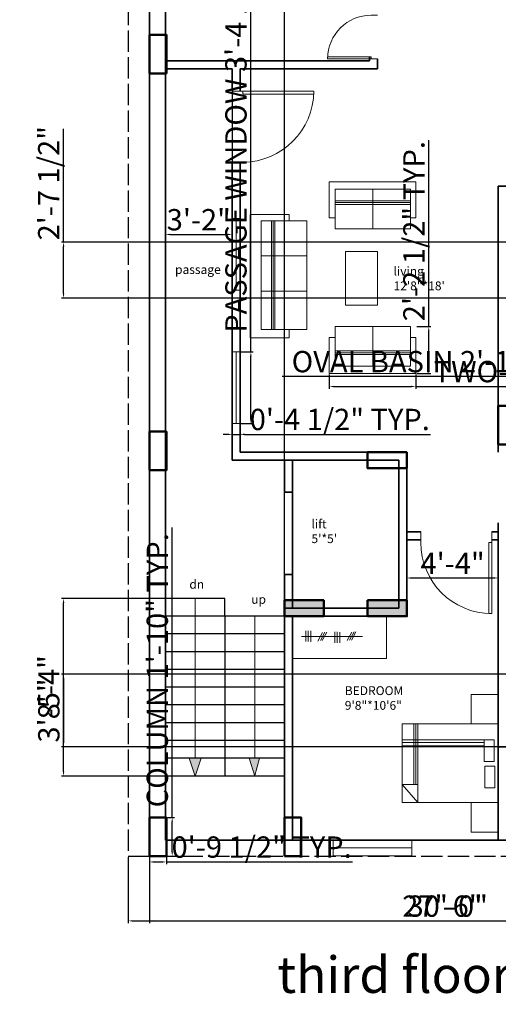
# Model space of a CAD drawing. Units: inches. Extents: x 2147 to 2722, y 2048 to 2905.
# Tile 1 of 3: x 2147 to 2417, y 2048 to 2602. Entities that reach past the tile are written whole.
import ezdxf

# ---------------------------------------------------------------- set-up
doc = ezdxf.new("R2010")
doc.units = ezdxf.units.IN
doc.linetypes.add('ACAD_ISO02W100', pattern=[15, 12, -3])
for name, color, linetype, lineweight in [('A-ANNO-DIMS', 2, 'Continuous', 18), ('A-ANNO-SYMB', 7, 'Continuous', 18), ('A-ANNO-TEXT', 7, 'Continuous', 18), ('A-ANNO-TITL', 7, 'Continuous', 35), ('A-AREA-IDEN', 7, 'Continuous', 18), ('A-COLS', 7, 'Continuous', 50), ('A-COLS-PATT', 252, 'Continuous', 13), ('A-DOOR', 3, 'Continuous', 18), ('A-FLOR-CASE', 8, 'Continuous', 18), ('A-FLOR-PATT', 252, 'Continuous', 13), ('A-FLOR-STRS', 7, 'Continuous', 25), ('A-FURN', 8, 'Continuous', 18), ('A-GLAZ', 4, 'Continuous', 18), ('A-WALL', 7, 'Continuous', 35), ('C-PROP', 6, 'ACAD_ISO02W100', 25)]:
    doc.layers.add(name, color=color, linetype=linetype, lineweight=lineweight)
doc.styles.get("Standard").update_dxf_attribs({"font": 'arial.ttf'})
doc.dimstyles.new('ISO-25', dxfattribs={"dimtxt": 12, "dimasz": 2.5, "dimexe": 1.25, "dimexo": 0.625, "dimtad": 1, "dimdec": 0, "dimlunit": 4, "dimtxsty": 'Standard', "dimcen": 2.5, "dimadec": 0, "dimazin": 0, "dimtfac": 1, "dimtdec": 0, "dimtmove": 0, "dimatfit": 3, "dimfxl": 1, "dimarcsym": 0})

# ---------------------------------------------------------------- blocks, each defined once
blk = doc.blocks.new('*U3')
for p, q in [((0, 0), (0, -6)), ((40, 0), (40, -6))]:
    blk.add_line(p, q)
blk.add_lwpolyline([(0, 0), (0, 40), (1.75, 40), (1.75, 0)], close=True)
blk.add_arc((0, 0), 40, 0, 90)
blk = doc.blocks.new('*D6')
at = {"layer": 'A-ANNO-DIMS', "color": 0, "lineweight": -2, "transparency": 16777216}
for p, q in [((2229.6, 2573.86), (2229.6, 2479.91)), ((2267.1, 2573.86), (2267.1, 2479.91)), ((2232.1, 2481.16), (2264.6, 2481.16))]:
    blk.add_line(p, q, dxfattribs=at)
at = {"layer": 'A-ANNO-DIMS', "color": 0, "lineweight": 100, "transparency": 16777216}
for points in [[(2232.1, 2481.58), (2232.1, 2480.74), (2229.6, 2481.16)], [(2264.6, 2481.58), (2264.6, 2480.74), (2267.1, 2481.16)]]:
    blk.add_solid(points, dxfattribs=at)
at = {"layer": 'Defpoints', "color": 0, "lineweight": 100, "transparency": 16777216}
for p in [(2229.6, 2574.49), (2267.1, 2574.49), (2267.1, 2481.16)]:
    blk.add_point(p, dxfattribs=at)
at = {"layer": 'A-ANNO-DIMS', "color": 0, "transparency": 16777216, "insert": (2248.35, 2487.92), "char_height": 12, "attachment_point": 5}
blk.add_mtext('3\'-2"', dxfattribs=at)
blk = doc.blocks.new('*D9')
at = {"layer": 'A-ANNO-DIMS', "color": 0, "lineweight": -2, "transparency": 16777216}
for p, q in [((2365.59, 2313.02), (2365.59, 2286.43)), ((2417.09, 2313.02), (2417.09, 2286.43)), ((2368.09, 2287.68), (2414.59, 2287.68))]:
    blk.add_line(p, q, dxfattribs=at)
at = {"layer": 'A-ANNO-DIMS', "color": 0, "lineweight": 100, "transparency": 16777216}
for points in [[(2368.09, 2288.1), (2368.09, 2287.27), (2365.59, 2287.68)], [(2414.59, 2288.1), (2414.59, 2287.27), (2417.09, 2287.68)]]:
    blk.add_solid(points, dxfattribs=at)
at = {"layer": 'Defpoints', "color": 0, "lineweight": 100, "transparency": 16777216}
for p in [(2365.59, 2313.64), (2417.09, 2313.64), (2417.09, 2287.68)]:
    blk.add_point(p, dxfattribs=at)
at = {"layer": 'A-ANNO-DIMS', "color": 0, "transparency": 16777216, "insert": (2391.34, 2294.31), "char_height": 12, "attachment_point": 5}
blk.add_mtext('4\'-4"', dxfattribs=at)
blk = doc.blocks.new('BED-TWIN-PILLOW')
for p, q in [((6.6, 10.17), (6.6, 44.18)), ((7.66, 10.17), (7.66, 44.18)), ((8.88, 10.17), (8.88, 44.18)), ((46.28, 35.34), (0, 35.34)), ((46.28, 33.66), (0, 33.66)), ((46.28, 31.83), (0, 31.83)), ((8.88, 0), (0, 10.17))]:
    blk.add_line(p, q)
for points in [[(54.22, 44.18), (0, 44.18), (0, 0), (54.22, 0)], [(51.93, 35.34), (46.28, 35.34), (46.28, 23.14), (51.93, 23.14)], [(52.24, 20.39), (46.59, 20.39), (46.59, 8.19), (52.24, 8.19)], [(0, 0), (8.88, 0), (8.88, 10.17), (0, 10.17)]]:
    blk.add_lwpolyline(points, close=True)
blk = doc.blocks.new('NIGHTSTAND')
blk.add_lwpolyline([(15.28, 0), (0, 0), (0, 16.69), (15.28, 16.69)], close=True)
blk = doc.blocks.new('SOFA-TWO-SEAT')
for p, q in [((24.52, 26.42), (24.52, 4.08)), ((3.35, 20.33), (0, 20.33)), ((0, 20.33), (0, 0)), ((48.72, 20.33), (45.68, 20.33)), ((48.72, 0), (48.72, 20.33)), ((3.35, 12.7), (45.68, 12.7)), ((3.35, 11.65), (45.68, 11.65)), ((3.35, 10.79), (45.68, 10.79)), ((0, 0), (48.72, 0))]:
    blk.add_line(p, q)
blk.add_lwpolyline([(3.35, 26.42), (45.68, 26.42), (45.68, 4.08), (3.35, 4.08)], close=True)
blk = doc.blocks.new('WINDOW-BEDROOM')
blk.add_line((0, 4.5), (44.35, 4.5))
blk.add_lwpolyline([(0, 9), (44.35, 9), (44.35, 0), (0, 0)], close=True)
blk = doc.blocks.new('WINDOW-PASSAGE')
blk.add_line((2.25, 0), (2.25, 40.45))
blk.add_lwpolyline([(0, 0), (4.5, 0), (4.5, 40.45), (0, 40.45)], close=True)
blk = doc.blocks.new('COLUMN-RECT')
blk.add_lwpolyline([(0, 0), (9.48, 0), (9.48, 21.75), (0, 21.75)], close=True)
blk = doc.blocks.new('*D26')
at = {"layer": 'A-ANNO-DIMS', "color": 0, "lineweight": -2, "transparency": 16777216}
for p, q in [((2233.34, 2152.74), (2233.34, 2316.12)), ((2230.7, 2152.74), (2234.59, 2152.74)), ((2233.34, 2133.49), (2233.34, 2150.24)), ((2230.7, 2130.99), (2234.59, 2130.99))]:
    blk.add_line(p, q, dxfattribs=at)
at = {"layer": 'A-ANNO-DIMS', "color": 0, "lineweight": 100, "transparency": 16777216}
for points in [[(2232.92, 2150.24), (2233.76, 2150.24), (2233.34, 2152.74)], [(2232.92, 2133.49), (2233.76, 2133.49), (2233.34, 2130.99)]]:
    blk.add_solid(points, dxfattribs=at)
at = {"layer": 'Defpoints', "color": 0, "lineweight": 100, "transparency": 16777216}
for p in [(2230.08, 2152.74), (2233.34, 2152.74), (2230.08, 2130.99)]:
    blk.add_point(p, dxfattribs=at)
at = {"layer": 'A-ANNO-DIMS', "color": 0, "transparency": 16777216, "insert": (2226.51, 2235.68), "char_height": 12, "attachment_point": 5, "rotation": 90}
blk.add_mtext('COLUMN 1\'-10" TYP.', dxfattribs=at)
blk = doc.blocks.new('*D27')
at = {"layer": 'A-ANNO-DIMS', "color": 0, "lineweight": -2, "transparency": 16777216}
for p, q in [((2220.6, 2130.36), (2220.6, 2126.48)), ((2230.08, 2130.36), (2230.08, 2126.48)), ((2223.1, 2127.73), (2227.58, 2127.73)), ((2230.08, 2127.73), (2334.94, 2127.73))]:
    blk.add_line(p, q, dxfattribs=at)
at = {"layer": 'A-ANNO-DIMS', "color": 0, "lineweight": 100, "transparency": 16777216}
for points in [[(2223.1, 2128.14), (2223.1, 2127.31), (2220.6, 2127.73)], [(2227.58, 2128.14), (2227.58, 2127.31), (2230.08, 2127.73)]]:
    blk.add_solid(points, dxfattribs=at)
at = {"layer": 'Defpoints', "color": 0, "lineweight": 100, "transparency": 16777216}
for p in [(2220.6, 2130.99), (2230.08, 2130.99), (2230.08, 2127.73)]:
    blk.add_point(p, dxfattribs=at)
at = {"layer": 'A-ANNO-DIMS', "color": 0, "transparency": 16777216, "insert": (2283.76, 2134.56), "char_height": 12, "attachment_point": 5}
blk.add_mtext('0\'-9 1/2" TYP.', dxfattribs=at)
blk = doc.blocks.new('*D30')
at = {"layer": 'A-ANNO-DIMS', "color": 0, "lineweight": -2, "transparency": 16777216}
for p, q in [((2476.51, 2404.28), (2476.51, 2399.9)), ((2501.53, 2404.28), (2501.53, 2399.9)), ((2476.51, 2401.15), (2295.38, 2401.15)), ((2499.03, 2401.15), (2479.01, 2401.15))]:
    blk.add_line(p, q, dxfattribs=at)
at = {"layer": 'A-ANNO-DIMS', "color": 0, "lineweight": 100, "transparency": 16777216}
for points in [[(2479.01, 2401.57), (2479.01, 2400.73), (2476.51, 2401.15)], [(2499.03, 2401.57), (2499.03, 2400.73), (2501.53, 2401.15)]]:
    blk.add_solid(points, dxfattribs=at)
at = {"layer": 'Defpoints', "color": 0, "lineweight": 100, "transparency": 16777216}
for p in [(2476.51, 2404.9), (2501.53, 2404.9), (2476.51, 2401.15)]:
    blk.add_point(p, dxfattribs=at)
at = {"layer": 'A-ANNO-DIMS', "color": 0, "transparency": 16777216, "insert": (2384.7, 2407.98), "char_height": 12, "attachment_point": 5}
blk.add_mtext('OVAL BASIN 2\'-1" TYP.', dxfattribs=at)
blk = doc.blocks.new('*D38')
at = {"layer": 'A-ANNO-DIMS', "color": 0, "lineweight": -2, "transparency": 16777216}
for p, q in [((2321.88, 2402.21), (2321.88, 2394.28)), ((2370.6, 2402.21), (2370.6, 2394.28)), ((2324.38, 2395.53), (2368.1, 2395.53)), ((2370.6, 2395.53), (2619.19, 2395.53))]:
    blk.add_line(p, q, dxfattribs=at)
at = {"layer": 'A-ANNO-DIMS', "color": 0, "lineweight": 100, "transparency": 16777216}
for points in [[(2324.38, 2395.95), (2324.38, 2395.11), (2321.88, 2395.53)], [(2368.1, 2395.95), (2368.1, 2395.11), (2370.6, 2395.53)]]:
    blk.add_solid(points, dxfattribs=at)
at = {"layer": 'Defpoints', "color": 0, "lineweight": 100, "transparency": 16777216}
for p in [(2321.88, 2402.84), (2370.6, 2402.84), (2370.6, 2395.53)]:
    blk.add_point(p, dxfattribs=at)
at = {"layer": 'A-ANNO-DIMS', "color": 0, "transparency": 16777216, "insert": (2496.15, 2402.36), "char_height": 12, "attachment_point": 5}
blk.add_mtext('TWO-SEAT SOFA 4\'-0 1/2" TYP.', dxfattribs=at)
blk = doc.blocks.new('*D39')
at = {"layer": 'A-ANNO-DIMS', "color": 0, "lineweight": -2, "transparency": 16777216}
for p, q in [((2377.91, 2429.26), (2377.91, 2534.32)), ((2371.23, 2429.26), (2379.16, 2429.26)), ((2377.91, 2405.34), (2377.91, 2426.76)), ((2371.23, 2402.84), (2379.16, 2402.84))]:
    blk.add_line(p, q, dxfattribs=at)
at = {"layer": 'A-ANNO-DIMS', "color": 0, "lineweight": 100, "transparency": 16777216}
for points in [[(2377.49, 2426.76), (2378.33, 2426.76), (2377.91, 2429.26)], [(2377.49, 2405.34), (2378.33, 2405.34), (2377.91, 2402.84)]]:
    blk.add_solid(points, dxfattribs=at)
at = {"layer": 'Defpoints', "color": 0, "lineweight": 100, "transparency": 16777216}
for p in [(2370.6, 2429.26), (2377.91, 2429.26), (2370.6, 2402.84)]:
    blk.add_point(p, dxfattribs=at)
at = {"layer": 'A-ANNO-DIMS', "color": 0, "transparency": 16777216, "insert": (2371.08, 2483.04), "char_height": 12, "attachment_point": 5, "rotation": 90}
blk.add_mtext('2\'-2 1/2" TYP.', dxfattribs=at)
blk = doc.blocks.new('*D44')
at = {"layer": 'A-ANNO-DIMS', "color": 0, "lineweight": -2, "transparency": 16777216}
for p, q in [((2277.67, 2415.1), (2277.67, 2682.36)), ((2272.22, 2415.1), (2278.92, 2415.1)), ((2277.67, 2377.15), (2277.67, 2412.6)), ((2272.22, 2374.65), (2278.92, 2374.65))]:
    blk.add_line(p, q, dxfattribs=at)
at = {"layer": 'A-ANNO-DIMS', "color": 0, "lineweight": 100, "transparency": 16777216}
for points in [[(2277.25, 2412.6), (2278.08, 2412.6), (2277.67, 2415.1)], [(2277.25, 2377.15), (2278.08, 2377.15), (2277.67, 2374.65)]]:
    blk.add_solid(points, dxfattribs=at)
at = {"layer": 'Defpoints', "color": 0, "lineweight": 100, "transparency": 16777216}
for p in [(2271.6, 2415.1), (2277.67, 2415.1), (2271.6, 2374.65)]:
    blk.add_point(p, dxfattribs=at)
at = {"layer": 'A-ANNO-DIMS', "color": 0, "transparency": 16777216, "insert": (2270.83, 2549.98), "char_height": 12, "attachment_point": 5, "rotation": 90}
blk.add_mtext('PASSAGE WINDOW 3\'-4 1/2" TYP.', dxfattribs=at)
blk = doc.blocks.new('*D45')
at = {"layer": 'A-ANNO-DIMS', "color": 0, "lineweight": -2, "transparency": 16777216}
for p, q in [((2267.1, 2374.02), (2267.1, 2367.33)), ((2271.6, 2374.02), (2271.6, 2367.33)), ((2264.6, 2368.58), (2262.1, 2368.58)), ((2267.1, 2368.58), (2271.6, 2368.58)), ((2274.1, 2368.58), (2378.95, 2368.58))]:
    blk.add_line(p, q, dxfattribs=at)
at = {"layer": 'A-ANNO-DIMS', "color": 0, "lineweight": 100, "transparency": 16777216}
for points in [[(2264.6, 2369), (2264.6, 2368.16), (2267.1, 2368.58)], [(2274.1, 2369), (2274.1, 2368.16), (2271.6, 2368.58)]]:
    blk.add_solid(points, dxfattribs=at)
at = {"layer": 'Defpoints', "color": 0, "lineweight": 100, "transparency": 16777216}
for p in [(2267.1, 2374.65), (2271.6, 2374.65), (2271.6, 2368.58)]:
    blk.add_point(p, dxfattribs=at)
at = {"layer": 'A-ANNO-DIMS', "color": 0, "transparency": 16777216, "insert": (2327.78, 2375.41), "char_height": 12, "attachment_point": 5}
blk.add_mtext('0\'-4 1/2" TYP.', dxfattribs=at)
blk = doc.blocks.new('*D46')
at = {"layer": 'A-ANNO-DIMS', "color": 0, "lineweight": -2, "transparency": 16777216}
for p, q in [((2208.6, 2130.36), (2208.6, 2093.29)), ((2568.6, 2130.36), (2568.6, 2093.29)), ((2211.1, 2094.54), (2566.1, 2094.54))]:
    blk.add_line(p, q, dxfattribs=at)
at = {"layer": 'A-ANNO-DIMS', "color": 0, "lineweight": 100, "transparency": 16777216}
for points in [[(2211.1, 2094.96), (2211.1, 2094.12), (2208.6, 2094.54)], [(2566.1, 2094.96), (2566.1, 2094.12), (2568.6, 2094.54)]]:
    blk.add_solid(points, dxfattribs=at)
at = {"layer": 'Defpoints', "color": 0, "lineweight": 100, "transparency": 16777216}
for p in [(2208.6, 2130.99), (2568.6, 2130.99), (2568.6, 2094.54)]:
    blk.add_point(p, dxfattribs=at)
at = {"layer": 'A-ANNO-DIMS', "color": 0, "transparency": 16777216, "insert": (2388.6, 2101.3), "char_height": 12, "attachment_point": 5}
blk.add_mtext('30\'-0"', dxfattribs=at)
blk = doc.blocks.new('*D47')
at = {"layer": 'A-ANNO-DIMS', "color": 0, "lineweight": -2, "transparency": 16777216}
for p, q in [((2220.6, 2130.36), (2220.6, 2093.29)), ((2550.6, 2130.51), (2550.6, 2093.29)), ((2223.1, 2094.54), (2548.1, 2094.54))]:
    blk.add_line(p, q, dxfattribs=at)
at = {"layer": 'A-ANNO-DIMS', "color": 0, "lineweight": 100, "transparency": 16777216}
for points in [[(2223.1, 2094.96), (2223.1, 2094.12), (2220.6, 2094.54)], [(2548.1, 2094.96), (2548.1, 2094.12), (2550.6, 2094.54)]]:
    blk.add_solid(points, dxfattribs=at)
at = {"layer": 'Defpoints', "color": 0, "lineweight": 100, "transparency": 16777216}
for p in [(2220.6, 2130.99), (2550.6, 2131.13), (2550.6, 2094.54)]:
    blk.add_point(p, dxfattribs=at)
at = {"layer": 'A-ANNO-DIMS', "color": 0, "transparency": 16777216, "insert": (2385.6, 2101.29), "char_height": 12, "attachment_point": 5}
blk.add_mtext('27\'-6"', dxfattribs=at)
blk = doc.blocks.new('*D48')
at = {"layer": 'A-ANNO-DIMS', "color": 0, "lineweight": -2, "transparency": 16777216}
for p, q in [((2229.6, 2266.77), (2229.6, 2768.69)), ((2232.1, 2767.44), (2294.09, 2767.44)), ((2296.59, 2266.77), (2296.59, 2768.69))]:
    blk.add_line(p, q, dxfattribs=at)
at = {"layer": 'A-ANNO-DIMS', "color": 0, "lineweight": 100, "transparency": 16777216}
for points in [[(2232.1, 2767.86), (2232.1, 2767.02), (2229.6, 2767.44)], [(2294.09, 2767.86), (2294.09, 2767.02), (2296.59, 2767.44)]]:
    blk.add_solid(points, dxfattribs=at)
at = {"layer": 'Defpoints', "color": 0, "lineweight": 100, "transparency": 16777216}
for p in [(2296.59, 2767.44), (2229.6, 2266.14), (2296.59, 2266.14)]:
    blk.add_point(p, dxfattribs=at)
at = {"layer": 'A-ANNO-DIMS', "color": 0, "transparency": 16777216, "insert": (2263.1, 2774.17), "char_height": 12, "attachment_point": 5}
blk.add_mtext('5\'-7"', dxfattribs=at)
blk = doc.blocks.new('*D49')
at = {"layer": 'A-ANNO-DIMS', "color": 0, "lineweight": -2, "transparency": 16777216}
for p, q in [((2228.97, 2276.14), (2170.9, 2276.14)), ((2172.15, 2178.64), (2172.15, 2273.64)), ((2228.97, 2176.14), (2170.9, 2176.14))]:
    blk.add_line(p, q, dxfattribs=at)
at = {"layer": 'A-ANNO-DIMS', "color": 0, "lineweight": 100, "transparency": 16777216}
for points in [[(2171.73, 2273.64), (2172.56, 2273.64), (2172.15, 2276.14)], [(2171.73, 2178.64), (2172.56, 2178.64), (2172.15, 2176.14)]]:
    blk.add_solid(points, dxfattribs=at)
at = {"layer": 'Defpoints', "color": 0, "lineweight": 100, "transparency": 16777216}
for p in [(2172.15, 2276.14), (2229.6, 2276.14), (2229.6, 2176.14)]:
    blk.add_point(p, dxfattribs=at)
at = {"layer": 'A-ANNO-DIMS', "color": 0, "transparency": 16777216, "insert": (2165.4, 2226.14), "char_height": 12, "attachment_point": 5, "rotation": 90}
blk.add_mtext('8\'-4"', dxfattribs=at)
blk = doc.blocks.new('*D50')
at = {"layer": 'A-ANNO-DIMS', "color": 0, "lineweight": -2, "transparency": 16777216}
for p, q in [((2486.75, 2233.45), (2170.9, 2233.45)), ((2172.15, 2230.95), (2172.15, 2195.13)), ((2483.59, 2192.63), (2170.9, 2192.63))]:
    blk.add_line(p, q, dxfattribs=at)
at = {"layer": 'A-ANNO-DIMS', "color": 0, "lineweight": 100, "transparency": 16777216}
for points in [[(2171.73, 2230.95), (2172.56, 2230.95), (2172.15, 2233.45)], [(2171.73, 2195.13), (2172.56, 2195.13), (2172.15, 2192.63)]]:
    blk.add_solid(points, dxfattribs=at)
at = {"layer": 'Defpoints', "color": 0, "lineweight": 100, "transparency": 16777216}
for p in [(2487.37, 2233.45), (2172.15, 2192.63), (2484.21, 2192.63)]:
    blk.add_point(p, dxfattribs=at)
at = {"layer": 'A-ANNO-DIMS', "color": 0, "transparency": 16777216, "insert": (2165.39, 2213.04), "char_height": 12, "attachment_point": 5, "rotation": 90}
blk.add_mtext('3\'-5"', dxfattribs=at)
blk = doc.blocks.new('*D51')
at = {"layer": 'A-ANNO-DIMS', "color": 0, "lineweight": -2, "transparency": 16777216}
for p, q in [((2172.15, 2476.87), (2172.15, 2540.69)), ((2452.47, 2476.87), (2170.9, 2476.87)), ((2172.15, 2447.87), (2172.15, 2474.37)), ((2452.47, 2445.37), (2170.9, 2445.37))]:
    blk.add_line(p, q, dxfattribs=at)
at = {"layer": 'A-ANNO-DIMS', "color": 0, "lineweight": 100, "transparency": 16777216}
for points in [[(2171.73, 2474.37), (2172.56, 2474.37), (2172.15, 2476.87)], [(2171.73, 2447.87), (2172.56, 2447.87), (2172.15, 2445.37)]]:
    blk.add_solid(points, dxfattribs=at)
at = {"layer": 'Defpoints', "color": 0, "lineweight": 100, "transparency": 16777216}
for p in [(2172.15, 2476.87), (2453.09, 2476.87), (2453.09, 2445.37)]:
    blk.add_point(p, dxfattribs=at)
at = {"layer": 'A-ANNO-DIMS', "color": 0, "transparency": 16777216, "insert": (2165.32, 2510.03), "char_height": 12, "attachment_point": 5, "rotation": 90}
blk.add_mtext('2\'-7 1/2"', dxfattribs=at)

msp = doc.modelspace()

# ---------------------------------------------------------------- hatches: boundary and pattern name
at = {"layer": 'A-COLS-PATT'}
h = msp.add_hatch(dxfattribs=at)
h.set_pattern_fill('AR-SAND', color=256, scale=5)
h.paths.add_polyline_path([(2439.24, 2712.96), (2417.09, 2712.96), (2417.09, 2703.96), (2421.59, 2703.96), (2421.59, 2703.99), (2439.24, 2703.99)])
h.paths.add_polyline_path([(2550.6, 2712.99), (2528.45, 2712.99), (2528.45, 2703.99), (2541.27, 2703.99), (2550.6, 2703.99)])
h.paths.add_polyline_path([(2229.6, 2593.61), (2220.6, 2593.61), (2220.6, 2571.86), (2229.6, 2571.86), (2229.6, 2574.49), (2230.08, 2574.49), (2230.08, 2578.99), (2229.6, 2578.99)])
h.paths.add_polyline_path([(2229.6, 2152.74), (2220.6, 2152.74), (2220.6, 2130.99), (2229.6, 2130.99), (2230.08, 2130.99), (2230.08, 2139.99), (2229.6, 2139.99)])
h.paths.add_polyline_path([(2301.09, 2152.74), (2296.59, 2152.74), (2296.59, 2140.02), (2301.09, 2140.03)])
h.paths.add_polyline_path([(2306.03, 2152.74), (2301.09, 2152.74), (2301.09, 2140.03), (2306.03, 2140.03)])
h.paths.add_polyline_path([(2306.03, 2140.03), (2296.55, 2140.02), (2296.55, 2130.99), (2306.03, 2130.99)])
h.paths.add_polyline_path([(2426.67, 2152.74), (2421.59, 2152.74), (2421.59, 2140.08), (2426.67, 2140.08)])
h.paths.add_polyline_path([(2421.59, 2152.74), (2417.19, 2152.74), (2417.19, 2140.08), (2421.59, 2140.08)])
h.paths.add_polyline_path([(2426.67, 2140.08), (2421.59, 2140.08), (2417.19, 2140.08), (2417.19, 2130.99), (2426.67, 2130.99)])
h = msp.add_hatch(dxfattribs=at)
h.set_pattern_fill('AR-SAND', color=256, scale=5)
h.paths.add_polyline_path([(2550.6, 2384.38), (2541.59, 2384.38), (2541.59, 2362.63), (2550.6, 2362.63)])
h.paths.add_polyline_path([(2426.57, 2384.56), (2421.59, 2384.56), (2421.59, 2367.13), (2426.57, 2367.13)], flags=17)
h.paths.add_polyline_path([(2421.59, 2384.56), (2417.09, 2384.56), (2417.09, 2362.81), (2426.57, 2362.81), (2426.57, 2367.13), (2421.59, 2367.13)])
h.paths.add_polyline_path([(2550.39, 2152.74), (2541.59, 2152.74), (2541.59, 2140.13), (2540.91, 2140.13), (2540.91, 2130.99), (2550.39, 2130.99)])
h.paths.add_polyline_path([(2361.09, 2353.99), (2343.4, 2353.99), (2343.4, 2349.49), (2361.09, 2349.49)], flags=17)
h.paths.add_polyline_path([(2365.55, 2358.49), (2343.4, 2358.49), (2343.4, 2353.99), (2361.09, 2353.99), (2361.09, 2349.49), (2365.55, 2349.49)])
h.paths.add_polyline_path([(2550.6, 2509.38), (2541.81, 2509.38), (2541.81, 2487.62), (2550.6, 2487.62)])
h.paths.add_polyline_path([(2229.6, 2370.15), (2220.6, 2370.15), (2220.6, 2348.39), (2229.6, 2348.39)])
h.paths.add_polyline_path([(2426.88, 2508.65), (2417.4, 2508.65), (2417.4, 2508.45), (2421.59, 2508.45), (2421.59, 2486.9), (2426.88, 2486.9)])
h.paths.add_polyline_path([(2421.59, 2508.45), (2417.4, 2508.45), (2417.4, 2486.9), (2421.59, 2486.9)], flags=17)
at = {"layer": 'A-FLOR-PATT'}
h = msp.add_hatch(color=256, dxfattribs=at)
h.dxf.hatch_style = 1
h.paths.add_polyline_path([(2249.6, 2186.14), (2246.35, 2186.14), (2242.96, 2186.14), (2246.35, 2176.14)])
h.paths.add_polyline_path([(2282.54, 2186.14), (2279.86, 2186.14), (2276.78, 2186.14), (2279.86, 2176.14), (2279.86, 2176.51)])
h.paths.add_polyline_path([(2318.74, 2275.14), (2301.09, 2275.14), (2301.09, 2270.63), (2318.74, 2270.63)])
h.paths.add_polyline_path([(2318.74, 2270.63), (2301.09, 2270.63), (2296.59, 2270.63), (2296.59, 2266.14), (2318.74, 2266.14)])
h.paths.add_polyline_path([(2301.09, 2275.14), (2296.59, 2275.14), (2296.59, 2270.63), (2301.09, 2270.63)])
h.paths.add_polyline_path([(2365.59, 2275.13), (2361.09, 2275.13), (2361.09, 2270.63), (2357.09, 2270.63), (2352.59, 2270.63), (2343.45, 2270.63), (2343.45, 2266.13), (2354.12, 2266.13), (2365.59, 2266.13)])
h.paths.add_polyline_path([(2361.09, 2275.13), (2343.45, 2275.13), (2343.45, 2270.63), (2352.59, 2270.63), (2357.09, 2270.63), (2361.09, 2270.63)], flags=17)

# ---------------------------------------------------------------- linework, layer by layer
at = {"layer": 'A-ANNO-SYMB'}
for p, q in [((2246.35, 2276.14), (2246.35, 2186.14)), ((2279.86, 2266.14), (2279.86, 2186.14)), ((2246.35, 2186.14), (2242.96, 2186.14)), ((2242.96, 2186.14), (2246.35, 2176.14)), ((2246.35, 2186.14), (2249.6, 2186.14)), ((2249.6, 2186.14), (2246.35, 2176.14)), ((2279.86, 2186.14), (2276.78, 2186.14)), ((2276.78, 2186.14), (2279.86, 2176.14)), ((2279.86, 2186.14), (2282.54, 2186.14)), ((2282.54, 2186.14), (2279.86, 2176.51)), ((2279.86, 2176.51), (2279.86, 2176.14))]:
    msp.add_line(p, q, dxfattribs=at)
at = {"layer": 'A-COLS'}
for points in [[(2417.09, 2362.81), (2426.57, 2362.81), (2426.57, 2384.56), (2417.09, 2384.56)], [(2220.6, 2348.39), (2230.08, 2348.39), (2230.08, 2370.15), (2220.6, 2370.15)], [(2343.4, 2358.49), (2365.55, 2358.49), (2365.55, 2349.49), (2343.4, 2349.49)], [(2296.59, 2275.14), (2318.74, 2275.14), (2318.74, 2266.14), (2296.59, 2266.14)], [(2343.45, 2275.13), (2365.59, 2275.13), (2365.59, 2266.13), (2343.45, 2266.13)]]:
    msp.add_lwpolyline(points, close=True, dxfattribs=at)
at = {"layer": 'A-FLOR-CASE'}
for p, q in [((2354.12, 2266.13), (2354.12, 2242.33)), ((2308.68, 2251.83), (2308.68, 2257.93)), ((2310.02, 2251.83), (2310.02, 2257.93)), ((2311.45, 2251.73), (2311.45, 2257.83)), ((2316.83, 2252.4), (2319.41, 2257.16)), ((2317.88, 2252.4), (2320.46, 2257.16)), ((2324.99, 2251.16), (2324.99, 2257.26)), ((2326.32, 2251.16), (2326.32, 2257.26)), ((2327.75, 2251.07), (2327.75, 2257.16)), ((2333.28, 2252.67), (2335.85, 2257.43)), ((2334.32, 2252.67), (2336.9, 2257.43)), ((2306.11, 2254.78), (2340.48, 2254.78)), ((2315.45, 2252.11), (2318.03, 2256.88)), ((2331.89, 2252.39), (2334.47, 2257.15))]:
    msp.add_line(p, q, dxfattribs=at)
msp.add_lwpolyline([(2354.12, 2266.13), (2301.09, 2266.13), (2301.09, 2242.33), (2354.12, 2242.33)], close=True, dxfattribs=at)
at = {"layer": 'A-FLOR-STRS'}
for p, q in [((2263.1, 2276.14), (2229.6, 2276.14)), ((2263.1, 2266.14), (2263.1, 2276.14)), ((2296.59, 2266.14), (2229.6, 2266.14)), ((2263.1, 2266.14), (2263.1, 2189.76)), ((2296.59, 2256.14), (2229.6, 2256.14)), ((2296.59, 2246.14), (2229.6, 2246.14)), ((2296.59, 2236.14), (2229.6, 2236.14)), ((2296.59, 2226.14), (2229.6, 2226.14)), ((2296.59, 2216.14), (2229.6, 2216.14)), ((2296.59, 2206.14), (2229.6, 2206.14)), ((2296.59, 2196.14), (2229.6, 2196.14)), ((2296.59, 2186.14), (2229.6, 2186.14)), ((2263.1, 2189.76), (2263.1, 2176.14)), ((2296.59, 2176.14), (2229.6, 2176.14))]:
    msp.add_line(p, q, dxfattribs=at)
at = {"layer": 'A-FURN'}
for p, q in [((2299.31, 2492.38), (2277.28, 2492.38)), ((2277.28, 2492.38), (2277.28, 2422.86)), ((2299.31, 2488.75), (2299.31, 2492.38)), ((2289.39, 2488.75), (2289.39, 2427.55)), ((2290.19, 2488.75), (2290.19, 2427.55)), ((2291.24, 2488.75), (2291.24, 2427.55)), ((2283.47, 2469.16), (2309.26, 2469.16)), ((2283.47, 2449.24), (2309.26, 2449.24)), ((2299.31, 2422.86), (2299.31, 2427.55)), ((2277.28, 2422.86), (2299.31, 2422.86))]:
    msp.add_line(p, q, dxfattribs=at)
for points in [[(2283.47, 2427.55), (2309.26, 2427.55), (2309.26, 2488.75), (2283.47, 2488.75)], [(2330.98, 2471.51), (2349.01, 2471.51), (2349.01, 2441.33), (2330.98, 2441.33)]]:
    msp.add_lwpolyline(points, close=True, dxfattribs=at)
at = {"layer": 'A-WALL'}
for p, q in [((2220.6, 2130.99), (2220.6, 2712.99)), ((2220.6, 2712.99), (2220.6, 2578.99)), ((2229.6, 2703.99), (2229.6, 2578.99)), ((2229.6, 2578.99), (2340.6, 2578.99)), ((2340.6, 2578.99), (2344.59, 2578.99)), ((2344.59, 2578.99), (2344.59, 2581.23)), ((2349.09, 2578.99), (2349.09, 2580.16)), ((2349.09, 2580.16), (2349.09, 2574.49)), ((2229.6, 2574.49), (2267.1, 2574.49)), ((2229.6, 2574.49), (2229.6, 2139.99)), ((2229.6, 2574.49), (2267.1, 2574.49)), ((2267.1, 2574.49), (2267.1, 2561.91)), ((2271.6, 2574.49), (2271.6, 2561.91)), ((2271.6, 2574.49), (2349.09, 2574.49)), ((2267.1, 2521.91), (2267.1, 2353.99)), ((2271.6, 2521.91), (2271.6, 2358.49)), ((2417.09, 2508.45), (2421.59, 2508.45)), ((2417.09, 2508.45), (2417.09, 2479.63)), ((2417.09, 2425.63), (2417.09, 2479.63)), ((2417.09, 2425.63), (2417.09, 2367.13)), ((2417.09, 2367.13), (2417.09, 2358.49)), ((2271.6, 2358.49), (2365.59, 2358.49)), ((2365.59, 2353.99), (2365.59, 2358.49)), ((2267.1, 2353.99), (2352.59, 2353.99)), ((2296.59, 2353.99), (2296.59, 2335.96)), ((2301.09, 2353.99), (2301.09, 2270.63)), ((2301.09, 2353.99), (2361.09, 2353.99)), ((2352.59, 2353.99), (2357.09, 2353.99)), ((2361.09, 2353.99), (2357.09, 2353.99)), ((2357.09, 2353.99), (2361.09, 2353.99)), ((2361.09, 2353.99), (2361.09, 2293.99)), ((2365.59, 2353.99), (2365.59, 2293.99)), ((2296.59, 2335.96), (2301.09, 2335.96)), ((2417.09, 2318.83), (2417.09, 2192.63)), ((2365.59, 2313.64), (2373.41, 2313.64)), ((2413.41, 2313.64), (2417.09, 2313.64)), ((2365.59, 2309.14), (2373.41, 2309.14)), ((2413.41, 2309.14), (2417.09, 2309.14)), ((2361.09, 2293.99), (2361.09, 2270.63)), ((2365.59, 2293.99), (2365.59, 2270.63)), ((2296.59, 2289.59), (2301.09, 2289.59)), ((2296.59, 2289.59), (2296.59, 2270.63)), ((2296.59, 2140.13), (2296.59, 2270.63)), ((2296.59, 2270.63), (2352.59, 2270.63)), ((2352.59, 2270.63), (2357.09, 2270.63)), ((2357.09, 2270.63), (2361.09, 2270.63)), ((2365.59, 2270.63), (2365.59, 2266.13)), ((2301.09, 2140.13), (2301.09, 2266.13)), ((2301.09, 2266.13), (2365.59, 2266.13)), ((2541.59, 2192.63), (2417.09, 2192.63)), ((2417.09, 2192.63), (2417.09, 2140.13)), ((2220.59, 2139.99), (2220.6, 2139.99)), ((2229.6, 2139.99), (2541.59, 2140.13)), ((2220.6, 2130.99), (2229.6, 2130.99)), ((2229.6, 2130.99), (2229.6, 2130.99))]:
    msp.add_line(p, q, dxfattribs=at)
at = {"layer": 'C-PROP'}
for p, q in [((2208.6, 2730.99), (2208.6, 2582.9)), ((2208.6, 2130.99), (2220.6, 2130.99))]:
    msp.add_line(p, q, dxfattribs=at)
msp.add_lwpolyline([(2208.6, 2130.99), (2568.6, 2130.99), (2568.6, 2730.99), (2208.6, 2730.99)], close=True, dxfattribs=at)

# ---------------------------------------------------------------- block references
at = {"layer": 'A-COLS'}
for p in [(2220.6, 2571.86), (2220.6, 2130.99), (2296.55, 2130.99)]:
    msp.add_blockref('COLUMN-RECT', p, dxfattribs=at)
at = {"layer": 'A-DOOR', "xscale": 0.6127871622533858, "yscale": 0.6127871622533858, "zscale": 0.6127871622533858, "rotation": 90.00000000000003}
msp.add_blockref('*U3', (2345.42, 2580.16), dxfattribs=at)
at = {"layer": 'A-DOOR'}
for p, rotation in [((2273.1, 2561.91), 270), ((2413.41, 2307.64), 180)]:
    msp.add_blockref('*U3', p, dxfattribs=dict(at, rotation=rotation))
at = {"layer": 'A-FURN', "extrusion": (0, 0, -1), "zscale": -1, "rotation": 180}
msp.add_blockref('SOFA-TWO-SEAT', (-2321.88, 2510.82), dxfattribs=at)
at = {"layer": 'A-FURN'}
for name, p in [('SOFA-TWO-SEAT', (2321.88, 2402.84)), ('NIGHTSTAND', (2401.82, 2205.44)), ('BED-TWIN-PILLOW', (2362.87, 2161.26)), ('NIGHTSTAND', (2401.82, 2144.57))]:
    msp.add_blockref(name, p, dxfattribs=at)
at = {"layer": 'A-GLAZ'}
for name, p in [('WINDOW-PASSAGE', (2267.1, 2449.73)), ('WINDOW-PASSAGE', (2267.1, 2374.65)), ('WINDOW-BEDROOM', (2324, 2131.12))]:
    msp.add_blockref(name, p, dxfattribs=at)

# ---------------------------------------------------------------- texts
at = {"layer": 'A-ANNO-TEXT', "char_height": 4.968, "attachment_point": 1}
for s, insert in [('dn', (2243.02, 2286.6)), ('up', (2277.89, 2278.1))]:
    msp.add_mtext_dynamic_manual_height_columns(s, width=78.277, gutter_width=24.84, heights=[0], dxfattribs=dict(at, insert=insert))
at = {"layer": 'A-ANNO-TITL', "insert": (2292.66, 2074.5), "char_height": 20.537, "attachment_point": 1}
msp.add_mtext_dynamic_manual_height_columns('third floor house plan', width=323.603, gutter_width=102.69, heights=[55.56], dxfattribs=at)
at = {"layer": 'A-AREA-IDEN', "char_height": 4.968, "attachment_point": 1}
for s, insert in [('passage', (2234.96, 2463.89)), ('living\\P12\'8"*18\'', (2358.04, 2462.98)), ("lift\\P5'*5'", (2311.8, 2320.59)), ('BEDROOM\\P9\'8"*10\'6"', (2330.59, 2226.7))]:
    msp.add_mtext_dynamic_manual_height_columns(s, width=78.277, gutter_width=24.84, heights=[0], dxfattribs=dict(at, insert=insert))

# ---------------------------------------------------------------- dimensions: what is measured, and where the dimension line sits
at = {"layer": 'A-ANNO-DIMS'}
for base, p1, p2, override, picture, middle in [((2296.59, 2767.44), (2229.6, 2266.14), (2296.59, 2266.14), {"dimdec": 1, "dimlfac": 1, "dimrnd": 0, "dimzin": 1, "dimdsep": 46, "dimlunit": 4, "dimfrac": 2}, '*D48', (2263.1, 2774.17)), ((2267.09701527, 2481.16103692), (2229.59701527, 2574.4898052), (2267.09701527, 2574.4898052), {"dimclrd": 0, "dimclre": 0, "dimclrt": 0}, '*D6', (2248.34701527, 2487.91700555)), ((2417.09358434, 2287.68210213), (2365.59358434, 2313.64195001), (2417.09358434, 2313.64195001), {"dimclrd": 0, "dimclre": 0, "dimclrt": 0}, '*D9', (2391.34358434, 2294.30710213)), ((2568.6, 2094.54), (2208.6, 2130.99), (2568.6, 2130.99), {"dimdec": 1, "dimlfac": 1, "dimrnd": 0, "dimzin": 1, "dimdsep": 46, "dimlunit": 4, "dimfrac": 2}, '*D46', (2388.6, 2101.3)), ((2550.6, 2094.54), (2220.6, 2130.99), (2550.6, 2131.13), {"dimdec": 1, "dimlfac": 1, "dimrnd": 0, "dimzin": 1, "dimdsep": 46, "dimlunit": 4, "dimfrac": 2}, '*D47', (2385.6, 2101.29))]:
    dim = msp.add_linear_dim(base=base, p1=p1, p2=p2, dimstyle='ISO-25', override=override, dxfattribs=at)
    dim.commit()
    dim.dimension.update_dxf_attribs({"geometry": picture, "text_midpoint": middle})
for base, p1, p2, angle, text, picture, middle in [((2277.6651, 2415.1016), (2271.597, 2374.6474), (2271.597, 2415.1016), 90, 'PASSAGE WINDOW <> TYP.', '*D44', (2270.8273, 2549.981)), ((2377.91, 2429.26), (2370.6, 2402.84), (2370.6, 2429.26), 90, '<> TYP.', '*D39', (2371.08, 2483.04)), ((2476.51, 2401.15), (2501.53, 2404.9), (2476.51, 2404.9), 180, 'OVAL BASIN <> TYP.', '*D30', (2384.7, 2407.98)), ((2233.3407, 2152.7406), (2230.0781, 2130.9898), (2230.0781, 2152.7406), 90, 'COLUMN <> TYP.', '*D26', (2226.507, 2235.6828))]:
    dim = msp.add_linear_dim(base=base, p1=p1, p2=p2, angle=angle, text=text, dimstyle='ISO-25', override={"dimdec": 1, "dimlfac": 1, "dimrnd": 0, "dimzin": 1, "dimdsep": 46, "dimlunit": 4, "dimfrac": 2}, dxfattribs=at)
    dim.commit()
    dim.dimension.update_dxf_attribs({"geometry": picture, "text_midpoint": middle})
for base, p1, p2, picture, middle in [((2172.15, 2476.87), (2453.09, 2445.37), (2453.09, 2476.87), '*D51', (2165.32, 2510.03)), ((2172.15, 2276.14), (2229.6, 2176.14), (2229.6, 2276.14), '*D49', (2165.4, 2226.14)), ((2172.15, 2192.63), (2487.37, 2233.45), (2484.21, 2192.63), '*D50', (2165.39, 2213.04))]:
    dim = msp.add_linear_dim(base=base, p1=p1, p2=p2, angle=90, dimstyle='ISO-25', override={"dimdec": 1, "dimlfac": 1, "dimrnd": 0, "dimzin": 1, "dimdsep": 46, "dimlunit": 4, "dimfrac": 2}, dxfattribs=at)
    dim.commit()
    dim.dimension.update_dxf_attribs({"geometry": picture, "text_midpoint": middle})
for base, p1, p2, text, picture, middle in [((2370.6, 2395.53), (2321.88, 2402.84), (2370.6, 2402.84), 'TWO-SEAT SOFA <> TYP.', '*D38', (2496.15, 2402.36)), ((2271.6, 2368.58), (2267.1, 2374.65), (2271.6, 2374.65), '<> TYP.', '*D45', (2327.78, 2375.41)), ((2230.08, 2127.73), (2220.6, 2130.99), (2230.08, 2130.99), '<> TYP.', '*D27', (2283.76, 2134.56))]:
    dim = msp.add_linear_dim(base=base, p1=p1, p2=p2, text=text, dimstyle='ISO-25', override={"dimdec": 1, "dimlfac": 1, "dimrnd": 0, "dimzin": 1, "dimdsep": 46, "dimlunit": 4, "dimfrac": 2}, dxfattribs=at)
    dim.commit()
    dim.dimension.update_dxf_attribs({"geometry": picture, "text_midpoint": middle})

doc.saveas('drawing.dxf')
